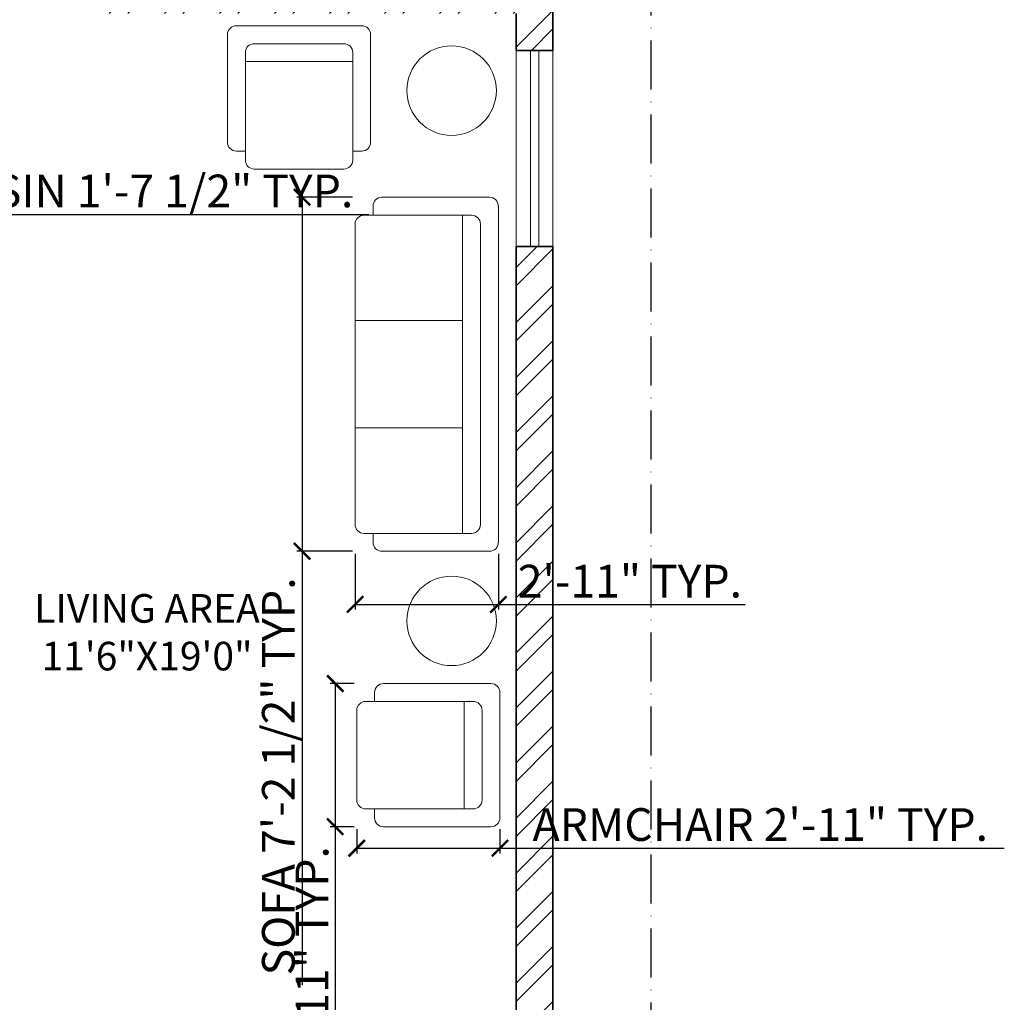
# Model space of a CAD drawing. Units: inches. Extents: x -15 to 1053, y -1 to 793.
# Tile 6 of 8: x 813 to 1053, y 256 to 496. Entities that reach past the tile are written whole.
import ezdxf

# ---------------------------------------------------------------- set-up
doc = ezdxf.new("R2010")
doc.units = ezdxf.units.IN
doc.linetypes.add('ACAD_ISO10W100', pattern=[18, 12, -3, 0, -3])
for name, color, linetype, lineweight in [('A-ANNO-DIMS', 2, 'Continuous', 18), ('A-AREA-IDEN', 7, 'Continuous', 18), ('A-FURN', 8, 'Continuous', 13), ('A-GLAZ', 4, 'Continuous', 18), ('A-WALL', 7, 'Continuous', 35), ('A-WALL-PATT', 8, 'Continuous', 13), ('C-PROP', 1, 'ACAD_ISO10W100', 25)]:
    doc.layers.add(name, color=color, linetype=linetype, lineweight=lineweight)
doc.styles.add('1-100DIM', font='txt', dxfattribs={"height": 0.3})
doc.styles.get("Standard").update_dxf_attribs({"font": 'arial.ttf'})
doc.dimstyles.new('ISO-25', dxfattribs={"dimtxt": 8, "dimasz": 4, "dimexe": 1.25, "dimexo": 0.625, "dimtad": 1, "dimdec": 0, "dimlunit": 4, "dimtxsty": 'Standard', "dimblk": 'ARCHTICK', "dimcen": 3, "dimadec": 0, "dimazin": 0, "dimtfac": 1, "dimtdec": 0, "dimtmove": 0, "dimatfit": 3, "dimldrblk": 'ARCHTICK', "dimfxl": 1, "dimarcsym": 0})

# ---------------------------------------------------------------- blocks, each defined once
blk = doc.blocks.new('sofa 6')
for p, q in [((-1044.4, 890), (1044.4, 890)), ((-1100, 166.9), (-1100, 834.3)), ((1100, 834.3), (1100, 166.9)), ((-933.1, 778.7), (933.1, 778.7)), ((-988.8, 55.6), (-988.8, 723.1)), ((988.8, 723.1), (988.8, 55.6)), ((-988.8, 667.5), (988.8, 667.5)), ((-333.8, 667.5), (-333.8, 0)), ((333.7, 667.5), (333.7, 0)), ((-988.8, 111.2), (-1044.4, 111.2)), ((1044.4, 111.2), (988.8, 111.2)), ((933.1, 0), (-933.1, 0))]:
    blk.add_line(p, q)
for centre, start, end in [((-1044.4, 834.3), 90, 180), ((1044.4, 834.3), 0, 90), ((-933.1, 723.1), 90, 180), ((933.1, 723.1), 0, 90), ((-1044.4, 166.9), 180, 270), ((1044.4, 166.9), 270, 0), ((-933.1, 55.6), 180, 270), ((933.1, 55.6), 270, 0)]:
    blk.add_arc(centre, 55.6, start, end)
blk = doc.blocks.new('ARMCHAIR')
for p, q in [((2.19, 30.66), (32.85, 30.66)), ((0, 2.19), (0, 28.47)), ((35.04, 28.47), (35.04, 2.19)), ((6.57, 26.28), (28.47, 26.28)), ((4.38, -2.19), (4.38, 24.09)), ((30.66, 24.09), (30.66, -2.19)), ((4.38, 0), (2.19, 0)), ((32.85, 0), (30.66, 0)), ((28.47, -4.38), (6.57, -4.38))]:
    blk.add_line(p, q)
for centre, start, end in [((2.19, 28.47), 90, 180), ((32.85, 28.47), 0, 90), ((6.57, 24.09), 90, 180), ((28.47, 24.09), 0, 90), ((2.19, 2.19), 180, 270), ((32.85, 2.19), 270, 0), ((6.57, -2.19), 180, 270), ((28.47, -2.19), 270, 0)]:
    blk.add_arc(centre, 2.19, start, end)
blk = doc.blocks.new('_ArchTick')
at = {"color": 0, "linetype": 'ByBlock', "const_width": 0.15}
blk.add_lwpolyline([(-0.5, -0.5), (0.5, 0.5)], dxfattribs=at)
blk = doc.blocks.new('*D40')
at = {"layer": 'A-ANNO-DIMS', "color": 0, "lineweight": -2, "transparency": 16777216}
for p, q in [((732.02, 450.92), (732.02, 447.33)), ((751.77, 450.92), (751.77, 447.33)), ((732.02, 448.58), (751.77, 448.58)), ((751.77, 448.58), (898.03, 448.58))]:
    blk.add_line(p, q, dxfattribs=at)
at = {"layer": 'Defpoints', "color": 0, "transparency": 16777216}
for p in [(732.02, 451.54), (751.77, 451.54), (751.77, 448.58)]:
    blk.add_point(p, dxfattribs=at)
at = {"layer": 'A-ANNO-DIMS', "color": 0, "lineweight": -2, "transparency": 16777216, "xscale": 4, "yscale": 4, "zscale": 4, "rotation": 180}
blk.add_blockref('_ArchTick', (732.02, 448.58), dxfattribs=at)
at = {"layer": 'A-ANNO-DIMS', "color": 0, "lineweight": -2, "transparency": 16777216, "xscale": 4, "yscale": 4, "zscale": 4}
blk.add_blockref('_ArchTick', (751.77, 448.58), dxfattribs=at)
at = {"layer": 'A-ANNO-DIMS', "color": 0, "transparency": 16777216, "insert": (826.9, 453.34), "char_height": 8, "attachment_point": 5}
blk.add_mtext('WASH BASIN 1\'-7 1/2" TYP.', dxfattribs=at)
blk = doc.blocks.new('*D46')
at = {"layer": 'A-ANNO-DIMS', "color": 0, "lineweight": -2, "transparency": 16777216}
for p, q in [((895.05, 298.21), (895.05, 292.33)), ((930.09, 298.21), (930.09, 292.33)), ((895.05, 293.58), (930.09, 293.58)), ((930.09, 293.58), (1053.49, 293.58))]:
    blk.add_line(p, q, dxfattribs=at)
at = {"layer": 'Defpoints', "color": 0, "transparency": 16777216}
for p in [(895.05, 298.84), (930.09, 298.84), (930.09, 293.58)]:
    blk.add_point(p, dxfattribs=at)
at = {"layer": 'A-ANNO-DIMS', "color": 0, "lineweight": -2, "transparency": 16777216, "xscale": 4, "yscale": 4, "zscale": 4, "rotation": 180}
blk.add_blockref('_ArchTick', (895.05, 293.58), dxfattribs=at)
at = {"layer": 'A-ANNO-DIMS', "color": 0, "lineweight": -2, "transparency": 16777216, "xscale": 4, "yscale": 4, "zscale": 4}
blk.add_blockref('_ArchTick', (930.09, 293.58), dxfattribs=at)
at = {"layer": 'A-ANNO-DIMS', "color": 0, "transparency": 16777216, "insert": (993.79, 298.34), "char_height": 8, "attachment_point": 5}
blk.add_mtext('ARMCHAIR 2\'-11" TYP.', dxfattribs=at)
blk = doc.blocks.new('*D47')
at = {"layer": 'A-ANNO-DIMS', "color": 0, "lineweight": -2, "transparency": 16777216}
for p, q in [((894.42, 333.87), (888.54, 333.87)), ((889.79, 333.87), (889.79, 298.84)), ((894.42, 298.84), (888.54, 298.84)), ((889.79, 298.84), (889.79, 238.47))]:
    blk.add_line(p, q, dxfattribs=at)
at = {"layer": 'Defpoints', "color": 0, "transparency": 16777216}
for p in [(895.05, 333.87), (889.79, 298.84), (895.05, 298.84)]:
    blk.add_point(p, dxfattribs=at)
at = {"layer": 'A-ANNO-DIMS', "color": 0, "lineweight": -2, "transparency": 16777216, "xscale": 4, "yscale": 4, "zscale": 4}
for p, rotation in [((889.79, 333.87), 90), ((889.79, 298.84), 270)]:
    blk.add_blockref('_ArchTick', p, dxfattribs=dict(at, rotation=rotation))
at = {"layer": 'A-ANNO-DIMS', "color": 0, "transparency": 16777216, "insert": (885.15, 266.65), "char_height": 8, "attachment_point": 5, "rotation": 90}
blk.add_mtext('2\'-11" TYP.', dxfattribs=at)
blk = doc.blocks.new('*D52')
at = {"layer": 'A-ANNO-DIMS', "color": 0, "lineweight": -2, "transparency": 16777216}
for p, q in [((894.04, 452.84), (880.42, 452.84)), ((881.67, 452.84), (881.67, 366.22)), ((894.04, 366.22), (880.42, 366.22)), ((881.67, 366.22), (881.67, 260.07))]:
    blk.add_line(p, q, dxfattribs=at)
at = {"layer": 'Defpoints', "color": 0, "transparency": 16777216}
for p in [(894.66, 452.84), (881.67, 366.22), (894.66, 366.22)]:
    blk.add_point(p, dxfattribs=at)
at = {"layer": 'A-ANNO-DIMS', "color": 0, "lineweight": -2, "transparency": 16777216, "xscale": 4, "yscale": 4, "zscale": 4}
for p, rotation in [((881.67, 452.84), 90), ((881.67, 366.22), 270)]:
    blk.add_blockref('_ArchTick', p, dxfattribs=dict(at, rotation=rotation))
at = {"layer": 'A-ANNO-DIMS', "color": 0, "transparency": 16777216, "insert": (876.91, 311.15), "char_height": 8, "attachment_point": 5, "rotation": 90}
blk.add_mtext('SOFA 7\'-2 1/2" TYP.', dxfattribs=at)
blk = doc.blocks.new('*D53')
at = {"layer": 'A-ANNO-DIMS', "color": 0, "lineweight": -2, "transparency": 16777216}
for p, q in [((894.66, 365.6), (894.66, 351.98)), ((929.7, 365.6), (929.7, 351.98)), ((894.66, 353.23), (929.7, 353.23)), ((929.7, 353.23), (990.07, 353.23))]:
    blk.add_line(p, q, dxfattribs=at)
at = {"layer": 'Defpoints', "color": 0, "transparency": 16777216}
for p in [(894.66, 366.22), (929.7, 366.22), (929.7, 353.23)]:
    blk.add_point(p, dxfattribs=at)
at = {"layer": 'A-ANNO-DIMS', "color": 0, "lineweight": -2, "transparency": 16777216, "xscale": 4, "yscale": 4, "zscale": 4, "rotation": 180}
blk.add_blockref('_ArchTick', (894.66, 353.23), dxfattribs=at)
at = {"layer": 'A-ANNO-DIMS', "color": 0, "lineweight": -2, "transparency": 16777216, "xscale": 4, "yscale": 4, "zscale": 4}
blk.add_blockref('_ArchTick', (929.7, 353.23), dxfattribs=at)
at = {"layer": 'A-ANNO-DIMS', "color": 0, "transparency": 16777216, "insert": (961.88, 357.88), "char_height": 8, "attachment_point": 5}
blk.add_mtext('2\'-11" TYP.', dxfattribs=at)

msp = doc.modelspace()

# ---------------------------------------------------------------- hatches: boundary and pattern name
at = {"layer": 'A-WALL-PATT'}
h = msp.add_hatch(dxfattribs=at)
h.set_pattern_fill('ANSI32', color=256)
h.paths.add_polyline_path([(754.07, 502.76), (754.07, 503.76), (652.07, 503.76), (652.07, 593.76), (643.07, 593.76), (643.07, 485.76), (652.07, 485.76), (652.07, 497.76), (754.07, 497.76)])
h.paths.add_polyline_path([(754.07, 449.76), (730.07, 449.76), (730.07, 467.76), (724.07, 467.76), (724.07, 449.76), (652.07, 449.76), (652.07, 461.76), (643.07, 461.76), (643.07, 374.76), (652.07, 374.76), (652.07, 443.76), (754.07, 443.76)])
h.paths.add_polyline_path([(757.07, 740.76), (643.07, 740.76), (643.07, 641.76), (652.07, 641.76), (652.07, 731.76), (700.07, 731.76), (700.07, 701.76), (706.07, 701.76), (706.07, 731.76), (757.07, 731.76)])
h.paths.add_polyline_path([(943.07, 740.76), (781.07, 740.76), (781.07, 731.76), (790.07, 731.76), (790.07, 671.76), (688.07, 671.76), (688.07, 665.76), (790.07, 665.76), (790.07, 497.76), (796.07, 497.76), (796.07, 502.76), (796.07, 731.76), (844.07, 731.76), (844.07, 701.76), (850.07, 701.76), (850.07, 731.76), (934.07, 731.76), (934.07, 713.76), (943.07, 713.76)])
h.paths.add_polyline_path([(943.07, 689.76), (934.07, 689.76), (934.07, 671.76), (832.07, 671.76), (832.07, 665.76), (934.07, 665.76), (934.07, 608.76), (943.07, 608.76)], flags=17)
h.paths.add_polyline_path([(943.07, 560.76), (934.07, 560.76), (934.07, 503.76), (832.07, 503.76), (832.07, 497.76), (934.07, 497.76), (934.07, 488.76), (943.07, 488.76)])
h.paths.add_polyline_path([(796.07, 449.76), (790.07, 449.76), (790.07, 444.76), (790.07, 326.76), (643.07, 326.76), (643.07, 320.76), (724.07, 320.76), (724.07, 266.76), (730.07, 266.76), (730.07, 320.76), (790.07, 320.76), (790.07, 272.76), (760.07, 272.76), (760.07, 266.76), (796.07, 266.76)])
h.paths.add_polyline_path([(652.07, 266.76), (688.07, 266.76), (688.07, 271.76), (688.07, 272.76), (643.07, 272.76), (643.07, 230.76), (652.07, 230.76)])
h.paths.add_polyline_path([(652.07, 182.76), (643.07, 182.76), (643.07, 146.76), (619.07, 146.76), (619.07, 44.76), (799.07, 44.76), (799.07, 53.76), (628.07, 53.76), (628.07, 137.76), (808.07, 137.76), (808.07, 146.76), (796.07, 146.76), (796.07, 218.76), (802.07, 218.76), (802.07, 224.76), (790.07, 224.76), (790.07, 146.76), (652.07, 146.76)])
h.paths.add_polyline_path([(886.07, 141.37), (886.07, 146.76), (850.07, 146.76), (850.07, 224.76), (838.07, 224.76), (838.07, 222.06), (838.07, 218.76), (844.07, 218.76), (844.07, 146.76), (832.07, 146.76), (832.07, 137.76), (886.07, 137.76)])
h.paths.add_polyline_path([(943.07, 176.76), (934.07, 176.76), (934.07, 137.76), (943.07, 137.76)])
h.paths.add_polyline_path([(943.07, 440.76), (934.07, 440.76), (934.07, 224.76), (943.07, 224.76)])

# ---------------------------------------------------------------- linework, layer by layer
at = {"layer": 'A-FURN'}
for p, q in [((894.08, 486.02), (867.8, 486.02)), ((921.33, 329.49), (921.33, 303.21))]:
    msp.add_line(p, q, dxfattribs=at)
for centre in [(918.26, 478.92), (918.26, 349.2)]:
    msp.add_circle(centre, 10.95, dxfattribs=at)
at = {"layer": 'A-GLAZ'}
for p, q in [((934.07, 488.76), (934.07, 440.76)), ((937.57, 488.76), (937.57, 440.76)), ((939.57, 488.76), (939.57, 440.76)), ((943.07, 488.76), (943.07, 440.76))]:
    msp.add_line(p, q, dxfattribs=at)
at = {"layer": 'A-WALL'}
for p, q in [((943.07, 488.76), (943.07, 560.76)), ((934.07, 488.76), (934.07, 497.76)), ((934.07, 488.76), (943.07, 488.76)), ((934.07, 440.76), (943.07, 440.76)), ((934.07, 224.76), (934.07, 440.76)), ((943.07, 224.76), (943.07, 440.76))]:
    msp.add_line(p, q, dxfattribs=at)
at = {"layer": 'C-PROP'}
msp.add_line((967.07, 44.76), (967.07, 764.76), dxfattribs=at)

# ---------------------------------------------------------------- block references
at = {"layer": 'A-FURN'}
msp.add_blockref('ARMCHAIR', (863.42, 464.12), dxfattribs=at)
at = {"layer": 'A-FURN', "xscale": 0.0393700787401575, "yscale": 0.0393700787401575, "zscale": 0.0393700787401575, "rotation": 270}
msp.add_blockref('sofa 6', (894.66, 409.53), dxfattribs=at)
at = {"layer": 'A-FURN', "rotation": 270.0000000001869}
msp.add_blockref('ARMCHAIR', (899.43, 333.87), dxfattribs=at)

# ---------------------------------------------------------------- texts
at = {"layer": 'A-AREA-IDEN', "insert": (801.39, 355.75), "char_height": 7, "attachment_point": 1, "style": '1-100DIM'}
msp.add_mtext_dynamic_manual_height_columns('\\pxqc;{\\f@Malgun Gothic|b0|i0|c0|p34;LIVING AREA\\P11\'6"X19\'0"}', width=84.7056, gutter_width=15.85, heights=[0], dxfattribs=at)

# ---------------------------------------------------------------- dimensions: what is measured, and where the dimension line sits
at = {"layer": 'A-ANNO-DIMS'}
for base, p1, p2, text, picture, middle in [((751.7657, 448.58), (732.02, 451.5418), (751.7657, 451.5418), 'WASH BASIN <> TYP.', '*D40', (826.8955, 453.3414)), ((929.7, 353.23), (894.66, 366.22), (929.7, 366.22), '<> TYP.', '*D53', (961.88, 357.88))]:
    dim = msp.add_linear_dim(base=base, p1=p1, p2=p2, text=text, dimstyle='ISO-25', override={"dimdec": 1, "dimrnd": 0, "dimzin": 1, "dimlunit": 4, "dimfrac": 2}, dxfattribs=at)
    dim.commit()
    dim.dimension.update_dxf_attribs({"geometry": picture, "text_midpoint": middle})
for base, p1, p2, angle, text, picture, middle in [((881.67, 366.22), (894.66, 452.84), (894.66, 366.22), 270, 'SOFA <> TYP.', '*D52', (876.91, 311.15)), ((889.79, 298.84), (895.05, 333.87), (895.05, 298.84), 270, '<> TYP.', '*D47', (885.15, 266.65)), ((930.09, 293.58), (895.05, 298.84), (930.09, 298.84), 0, 'ARMCHAIR <> TYP.', '*D46', (993.79, 298.34))]:
    dim = msp.add_linear_dim(base=base, p1=p1, p2=p2, angle=angle, text=text, dimstyle='ISO-25', override={"dimdec": 1, "dimrnd": 0, "dimzin": 1, "dimlunit": 4, "dimfrac": 2}, dxfattribs=at)
    dim.commit()
    dim.dimension.update_dxf_attribs({"geometry": picture, "text_midpoint": middle})

doc.saveas('drawing.dxf')
